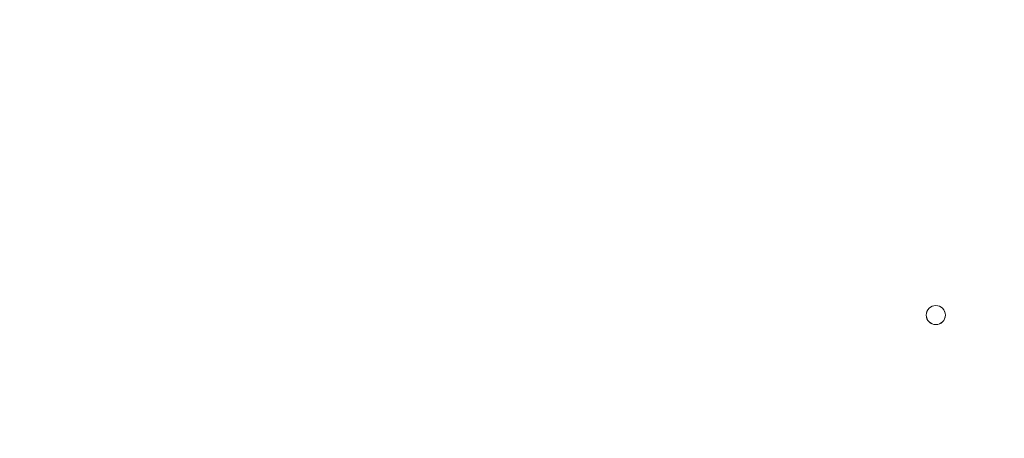
# Model space of a CAD drawing. Units: inches. Extents: x -466983 to 1020, y 324 to 318697.
# Tile 56 of 97: x 637.858 to 643.839, y 936.436 to 938.98. Entities that reach past the tile are written whole.
import ezdxf

# ---------------------------------------------------------------- set-up
doc = ezdxf.new("R2010")
doc.units = ezdxf.units.IN
doc.header["$MEASUREMENT"] = 0
doc.layers.add('A-FLOR-PATT', color=252, linetype='Continuous', lineweight=13)
doc.layers.add('A-FURN', color=8, linetype='Continuous', lineweight=18)

# ---------------------------------------------------------------- blocks, each defined once
blk = doc.blocks.new('L Shaped Sofa')
at = {"ltscale": 2}
for start, end in [(90, 270), (270, 90)]:
    blk.add_arc((2419.413, 753.788), 0.106, start, end, dxfattribs=at)

msp = doc.modelspace()

# ---------------------------------------------------------------- hatches: boundary and pattern name
at = {"layer": 'A-FLOR-PATT', "transparency": 33554572}
h = msp.add_hatch(dxfattribs=at)
h.set_pattern_fill('ANSI37', color=256, scale=30)
h.set_pattern_definition([(45, (-1212.4137, -290.035), (-2.6516504, 2.6516504), []), (135, (-1212.4137, -290.035), (-2.6516504, -2.6516504), [])])
h.paths.add_polyline_path([(901.8057, 1075.9377), (900.6144, 1075.9377), (900.6144, 1065.3856), (899.391, 1065.3856), (898.0911, 1065.3856), (892.8356, 1058.7098, -0.258377), (892.1875, 1058.3509), (879.9848, 1058.3509, -0.20177), (879.4382, 1058.5808), (874.0812, 1065.3856), (872.7813, 1065.3856), (871.5579, 1065.3856), (871.5579, 1075.9377), (813.8057, 1075.9377), (813.8057, 1044.7922), (832.3947, 1044.7922, -0.394795), (848.6602, 1028.5356), (848.6602, 1009.9377), (901.8057, 1009.9377), (901.8057, 1015.9377), (901.3057, 1015.9377), (871.3057, 1015.9377), (871.3057, 1017.2502), (871.3344, 1017.2502, -0.401453), (901.3057, 1045.9377), (901.8057, 1045.9377)])
edge = h.paths.add_edge_path(flags=16)
edge.add_line((847.7731, 1068.9486), (847.7731, 1073.7088))
edge.add_arc((849.2269, 1073.7088), 1.4538, 90, 180, ccw=False)
edge.add_line((849.2269, 1075.1627), (864.4921, 1075.1627))
edge.add_arc((864.4921, 1073.7088), 1.4538, 0, 90, ccw=False)
edge.add_line((865.9459, 1073.7088), (865.9459, 1069.0035))
edge.add_arc((832.6447, 1068.9761), 33.3012, -20.61234, 0.04725, ccw=False)
edge.add_ellipse((856.8595, 1058.48), major_axis=(0, 10.2131), ratio=0.6859192, start_angle=100.00884, end_angle=259.99116, ccw=False)
edge.add_arc((881.0742, 1068.9761), 33.3012, 180.04725, 200.61234, ccw=False)
h.paths.add_polyline_path([(853.1456, 1066.4815), (853.1456, 1066.4534), (853.1463, 1066.4534, 0.433107), (852.9166, 1066.6849), (852.9166, 1066.4534), (853.1456, 1066.4534), (853.1456, 1066.4815), (853.088, 1066.6122, 0.697939), (852.6995, 1066.4534), (852.7003, 1066.4534), (852.7003, 1066.4815), (852.9166, 1067.0012), (852.9166, 1066.6849, -0.396254)], flags=0)
h.paths.add_polyline_path([(861.0187, 1066.4815), (861.0187, 1066.4534), (861.0194, 1066.4534, 0.416404), (860.8024, 1066.6849), (860.8024, 1066.4534), (861.0187, 1066.4534), (861.0187, 1066.4815), (860.9672, 1066.6053, 0.713344), (860.5726, 1066.4534), (860.5734, 1066.4534), (860.5734, 1066.4815), (860.8024, 1067.0012), (860.8024, 1066.6849, -0.379973)], flags=0)
edge = h.paths.add_edge_path(flags=0)
edge.add_spline(control_points=[(861.1298, 1065.7855), (861.4661, 1065.2478), (861.6134, 1065.0161), (861.9833, 1064.3736), (862.1924, 1063.9443), (862.5614, 1063.0391), (862.7212, 1062.5633), (862.9865, 1061.5781), (863.092, 1061.0689), (863.2452, 1060.031), (863.293, 1059.5025), (863.3295, 1058.4409), (863.3181, 1057.9078), (863.2366, 1056.8518), (863.1664, 1056.3289), (862.9695, 1055.308), (862.8427, 1054.8099), (862.5365, 1053.8522), (862.3571, 1053.3927), (861.9514, 1052.5249), (861.7251, 1052.1166), (861.233, 1051.3622), (860.9672, 1051.0162), (860.4048, 1050.3949), (860.1082, 1050.1197), (859.4937, 1049.6461), (859.1758, 1049.4476), (858.5276, 1049.1299), (858.1973, 1049.0107), (857.5315, 1048.8518), (857.1959, 1048.8121), (856.5249, 1048.812), (856.1894, 1048.8515), (855.5236, 1049.0101), (855.1933, 1049.1291), (854.545, 1049.4465), (854.2271, 1049.6449), (853.6124, 1050.1183), (853.3158, 1050.3933), (852.7533, 1051.0143), (852.4874, 1051.3602), (851.9952, 1052.1144), (851.7688, 1052.5225), (851.3629, 1053.3902), (851.1834, 1053.8496), (850.877, 1054.8071), (850.7501, 1055.3051), (850.553, 1056.326), (850.4827, 1056.8488), (850.401, 1057.9048), (850.3895, 1058.4379), (850.4257, 1059.4995), (850.4734, 1060.0281), (850.6265, 1061.066), (850.7318, 1061.5753), (850.9969, 1062.5605), (851.1567, 1063.0365), (851.5254, 1063.9418), (851.7345, 1064.3712), (852.1056, 1065.0164), (852.2544, 1065.2503), (852.6082, 1065.7335)], knot_values=[3.915332, 3.915332, 3.915332, 3.915332, 4.013468, 4.013468, 4.175532, 4.175532, 4.337596, 4.337596, 4.49966, 4.49966, 4.661724, 4.661724, 4.823788, 4.823788, 4.985852, 4.985852, 5.147916, 5.147916, 5.30998, 5.30998, 5.472044, 5.472044, 5.634109, 5.634109, 5.796173, 5.796173, 5.958237, 5.958237, 6.120301, 6.120301, 6.282365, 6.282365, 6.444429, 6.444429, 6.606493, 6.606493, 6.768557, 6.768557, 6.930621, 6.930621, 7.092685, 7.092685, 7.254749, 7.254749, 7.416813, 7.416813, 7.578878, 7.578878, 7.740942, 7.740942, 7.903006, 7.903006, 8.06507, 8.06507, 8.227134, 8.227134, 8.389198, 8.389198, 8.551262, 8.551262, 8.65037, 8.65037, 8.65037, 8.65037], degree=3, periodic=0)
edge.add_line((852.6421, 1065.7855), (861.1298, 1065.7855))
edge = h.paths.add_edge_path(flags=0)
edge.add_ellipse((856.8496, 1057.7432), major_axis=(0, 7.7921), ratio=0.687861, start_angle=0, end_angle=360)
h.paths.add_polyline_path([(848.8634, 1069.3891), (848.8634, 1073.9605, -0.414214), (849.9538, 1075.0508), (863.7652, 1075.0508, -0.414214), (864.8555, 1073.9605), (864.8555, 1069.3891, -0.388936), (864.5237, 1069.027, -0.043561), (849.1953, 1069.027, -0.388936)], flags=0)
h.paths.add_polyline_path([(853.1006, 1068.1122, -1), (852.6775, 1068.1122, -1)], flags=0)
edge = h.paths.add_edge_path(flags=0)
edge.add_ellipse((856.8595, 1057.3378), major_axis=(0, 2.207), ratio=0.657164, start_angle=0, end_angle=360)
h.paths.add_polyline_path([(861.0415, 1068.1122, -1), (860.6184, 1068.1122, -1)], flags=0)
edge = h.paths.add_edge_path()
edge.add_line((573.9537, 1057.3412), (573.9537, 1075.9377))
edge.add_line((573.9537, 1075.9377), (558.7308, 1075.9377))
edge.add_line((558.7308, 1075.9377), (558.7308, 1065.3856))
edge.add_line((558.7308, 1065.3856), (557.5074, 1065.3856))
edge.add_line((557.5074, 1065.3856), (556.2075, 1065.3856))
edge.add_line((556.2075, 1065.3856), (550.952, 1058.7098))
edge.add_arc((550.3039, 1059.1155), 0.7646, 270, 327.94832, ccw=False)
edge.add_line((550.3039, 1058.3509), (538.1012, 1058.3509))
edge.add_arc((538.1012, 1059.1155), 0.7646, 224.3704, 270, ccw=False)
edge.add_line((537.5546, 1058.5808), (532.1976, 1065.3856))
edge.add_line((532.1976, 1065.3856), (530.8977, 1065.3856))
edge.add_line((530.8977, 1065.3856), (529.6743, 1065.3856))
edge.add_line((529.6743, 1065.3856), (529.6743, 1075.9377))
edge.add_line((529.6743, 1075.9377), (520.8057, 1075.9377))
edge.add_line((520.8057, 1075.9377), (520.8057, 1045.9377))
edge.add_line((520.8057, 1045.9377), (521.3057, 1045.9377))
edge.add_arc((521.3057, 1015.9377), 30, 2.50749, 90, ccw=False)
edge.add_line((551.277, 1017.2502), (551.3057, 1017.2502))
edge.add_line((551.3057, 1017.2502), (551.3057, 1015.9377))
edge.add_line((551.3057, 1015.9377), (520.8057, 1015.9377))
edge.add_line((520.8057, 1015.9377), (520.8057, 1009.9377))
edge.add_line((520.8057, 1009.9377), (559.1913, 1010.4022))
edge.add_arc((559.1913, 1011.856), 1.4538, 180, 270, ccw=False)
edge.add_line((557.7375, 1011.856), (557.7375, 1016.5613))
edge.add_arc((591.0386, 1016.5888), 33.3012, 159.38766, 180.04725, ccw=False)
edge.add_ellipse((566.8239, 1027.0848), major_axis=(0, 10.2131), ratio=0.6859192, start_angle=280.00884, end_angle=439.99116, ccw=False)
edge.add_arc((542.6091, 1016.5888), 33.3012, 0.04725, 20.61234, ccw=False)
edge.add_line((575.9103, 1016.6162), (575.9103, 1011.856))
edge.add_arc((574.4565, 1011.856), 1.4538, -90, 0, ccw=False)
edge.add_line((574.4565, 1010.4022), (608.8057, 1009.9377))
edge.add_line((608.8057, 1009.9377), (608.8057, 1041.0857))
edge.add_line((608.8057, 1041.0857), (590.2179, 1041.0857))
edge.add_arc((590.775, 1057.9074), 16.8309, 181.92775, 268.10321, ccw=False)
edge = h.paths.add_edge_path()
edge.add_ellipse((494.2443, 583.6204), major_axis=(0, 10.2131), ratio=0.6859192, start_angle=280.00884, end_angle=439.99116, ccw=False)
edge.add_arc((470.0296, 573.1243), 33.3012, 0.04725, 20.61234, ccw=False)
edge.add_line((503.3307, 573.1518), (503.3307, 568.3916))
edge.add_arc((501.8769, 568.3916), 1.4538, -90, 0, ccw=False)
edge.add_line((501.8769, 566.9377), (539.8057, 566.9377))
edge.add_line((539.8057, 566.9377), (539.8057, 572.9377))
edge.add_line((539.8057, 572.9377), (539.3057, 572.9377))
edge.add_line((539.3057, 572.9377), (509.3057, 572.9377))
edge.add_line((509.3057, 572.9377), (509.3057, 574.2502))
edge.add_line((509.3057, 574.2502), (509.3344, 574.2502))
edge.add_arc((539.3057, 572.9377), 30, 90, 177.49251, ccw=False)
edge.add_line((539.3057, 602.9377), (539.8057, 602.9377))
edge.add_line((539.8057, 602.9377), (539.8057, 626.9377))
edge.add_line((539.8057, 626.9377), (531.7718, 626.9377))
edge.add_line((531.7718, 626.9377), (531.7718, 616.3856))
edge.add_line((531.7718, 616.3856), (530.5484, 616.3856))
edge.add_line((530.5484, 616.3856), (529.2485, 616.3856))
edge.add_line((529.2485, 616.3856), (523.7105, 609.3509))
edge.add_line((523.7105, 609.3509), (510.7766, 609.3509))
edge.add_line((510.7766, 609.3509), (505.2386, 616.3856))
edge.add_line((505.2386, 616.3856), (503.9387, 616.3856))
edge.add_line((503.9387, 616.3856), (502.7153, 616.3856))
edge.add_line((502.7153, 616.3856), (502.7153, 626.9377))
edge.add_line((502.7153, 626.9377), (481.6983, 626.9377))
edge.add_line((481.6983, 626.9377), (481.6983, 610.995))
edge.add_arc((467.2703, 611.4728), 14.4359, 271.92775, 358.10321, ccw=False)
edge.add_line((467.7559, 597.0451), (451.8057, 597.0451))
edge.add_line((451.8057, 597.0451), (451.8057, 584.4035))
edge.add_line((451.8057, 584.4035), (451.8057, 566.9377))
edge.add_line((451.8057, 566.9377), (486.6117, 566.9377))
edge.add_arc((486.6117, 568.3916), 1.4538, 180, 270, ccw=False)
edge.add_line((485.1579, 568.3916), (485.1579, 573.0969))
edge.add_arc((518.4591, 573.1243), 33.3012, 159.38766, 180.04725, ccw=False)
h.paths.add_polyline_path([(836.2609, 1020.7328), (879.8898, 1020.7328), (879.8898, 1039.3902), (836.2609, 1039.3902)], flags=25)
h.paths.add_polyline_path([(549.9851, 1036.7492), (593.614, 1036.7492), (593.614, 1055.4065), (549.9851, 1055.4065)], flags=24)
h.paths.add_polyline_path([(475.123, 595.5959), (518.752, 595.5959), (518.752, 614.2532), (475.123, 614.2532)], flags=24)
h = msp.add_hatch(dxfattribs=at)
h.set_pattern_fill('ANSI37', color=256, scale=20)
h.set_pattern_definition([(45, (-1212.4137, -290.035), (-1.767767, 1.767767), []), (135, (-1212.4137, -290.035), (-1.767767, -1.767767), [])])
h.paths.add_polyline_path([(809.8057, 870.9377), (809.8057, 888.1519), (806.9985, 888.1519), (802.6624, 888.1519), (789.3832, 888.1519), (786.2846, 888.1519, -0.414214), (785.4991, 888.9374), (785.4991, 900.1959), (785.4991, 908.4696, -0.414214), (786.8082, 909.7787, -0.414214), (785.4991, 911.0878), (785.4991, 929.1015, -0.414214), (786.8082, 930.4106, -0.414214), (785.4991, 931.7197), (785.4991, 931.9039, -0.414214), (784.19, 930.5948), (766.7223, 930.5948, -0.412359), (765.4132, 931.8956, -0.413741), (764.1145, 930.5782), (744.5781, 930.422, -0.416556), (743.7864, 931.2075), (743.7864, 933.5153), (742.2154, 933.5153), (742.2154, 952.024, -0.001344), (743.7864, 952.1998), (743.7864, 953.9377), (678.5915, 953.9377), (678.5915, 951.1305), (678.5915, 946.7945), (678.5915, 933.5153), (678.5915, 930.4166, -0.414214), (677.806, 929.6312), (666.5475, 929.6312), (658.2738, 929.6312, -0.414214), (656.9647, 930.9403, -0.414214), (655.6556, 929.6312), (637.6419, 929.6312, -0.414214), (636.3328, 930.9403, -0.414214), (635.0237, 929.6312), (634.8395, 929.6312, -0.414214), (636.1486, 928.322), (636.1486, 910.8544, -0.412359), (634.8478, 909.5452, -0.413741), (636.1653, 908.2466), (636.3214, 888.7102, -0.416556), (635.5359, 887.9184), (633.2281, 887.9184), (633.2281, 886.3475), (614.7194, 886.3475, -0.001344), (614.5436, 887.9184), (612.8057, 887.9184), (612.8057, 834.9377), (612.8057, 752.9377), (612.8057, 748.9377), (612.8057, 697.9377), (654.8057, 697.9377), (654.8057, 701.9377), (715.8057, 701.9377), (715.8057, 737.4353), (774.2918, 737.4353), (774.2918, 795.9377), (809.8057, 795.9377)])
h.paths.add_polyline_path([(679.2761, 849.5757, 0.102523), (682.1475, 849.2608, -0.080461), (694.5428, 849.7725, -0.283899), (694.4822, 849.0082, 0.136605), (694.4068, 848.8103, -0.030441), (694.5428, 846.8929), (694.5428, 842.6198), (694.5428, 838.3466, -0.028219), (694.4246, 836.5684), (694.425, 836.5684, 0.196187), (694.4456, 836.2708, -0.302897), (694.5428, 835.467, -0.080461), (682.1475, 835.9787, 0.102523), (679.2761, 835.6638, -0.58611), (678.6457, 836.0169), (678.6457, 849.2227, -0.58611)], flags=16)
h.paths.add_polyline_path([(679.5173, 848.6515, 0.699597), (679.476, 848.6342, 1.20716), (679.1935, 848.7422, 0.010621)], flags=0)
h.paths.add_polyline_path([(679.4923, 836.5608, -0.013798), (679.9178, 836.6594, -0.071703), (682.8533, 837.1434, -0.165743), (682.1665, 839.1006), (682.1665, 842.6094), (682.1665, 846.0603, -0.240616), (683.4733, 848.6767, -0.068263), (693.9295, 849.0082), (693.7875, 848.7083), (693.7875, 849.0228, 0.067332), (683.4733, 848.6767, 0.240616), (682.1665, 846.0603), (682.1665, 842.6094), (682.1665, 839.1006, 0.23459), (683.461, 836.5513, 0.068093), (693.7875, 836.1955), (693.7875, 836.5104), (693.9296, 836.2102, -0.077215), (682.2421, 836.7815, 0.086627), (679.5283, 836.5701, -0.628402), (679.5029, 836.5735), (679.5029, 836.6071, 0.910458)], flags=0)
h.paths.add_polyline_path([(679.476, 848.6364), (679.2069, 848.647), (679.2069, 836.5718, 0.913566), (679.3645, 836.5861), (679.476, 836.5824)], flags=0)
h.paths.add_polyline_path([(679.2761, 829.8604, 0.102523), (682.1475, 829.5455, -0.080461), (694.5428, 830.0572, -0.283899), (694.4822, 829.2929, 0.136605), (694.4068, 829.095, -0.030441), (694.5428, 827.1776), (694.5428, 822.9045), (694.5428, 818.6314, -0.028219), (694.4246, 816.8531), (694.425, 816.8532, 0.196187), (694.4456, 816.5555, -0.302897), (694.5428, 815.7517, -0.080461), (682.1475, 816.2635, 0.102523), (679.2761, 815.9485, -0.58611), (678.6457, 816.3016), (678.6457, 829.5074, -0.58611)], flags=16)
h.paths.add_polyline_path([(679.5173, 828.9362, 0.699597), (679.476, 828.9189, 1.20716), (679.1935, 829.0269, 0.010621)], flags=0)
h.paths.add_polyline_path([(679.4923, 816.8456, -0.013798), (679.9178, 816.9441, -0.071703), (682.8533, 817.4281, -0.165743), (682.1665, 819.3853), (682.1665, 822.8941), (682.1665, 826.345, -0.240616), (683.4733, 828.9614, -0.068263), (693.9295, 829.2929), (693.7875, 828.9931), (693.7875, 829.3076, 0.067332), (683.4733, 828.9614, 0.240616), (682.1665, 826.345), (682.1665, 822.8941), (682.1665, 819.3853, 0.23459), (683.461, 816.836, 0.068093), (693.7875, 816.4802), (693.7875, 816.7952), (693.9296, 816.4949, -0.077215), (682.2421, 817.0662, 0.086627), (679.5283, 816.8549, -0.628402), (679.5029, 816.8582), (679.5029, 816.8918, 0.910458)], flags=0)
h.paths.add_polyline_path([(679.476, 828.9211), (679.2069, 828.9317), (679.2069, 816.8565, 0.913566), (679.3645, 816.8708), (679.476, 816.8671)], flags=0)
h.paths.add_polyline_path([(679.2761, 810.1451, 0.102523), (682.1475, 809.8302, -0.080461), (694.5428, 810.342, -0.3023), (694.4466, 809.5394, 0.10023), (694.4058, 809.3878, -0.03057), (694.5428, 807.4623), (694.5428, 803.1892), (694.5428, 798.9161, -0.03057), (694.4058, 796.9906, 0.10023), (694.4466, 796.839, -0.3023), (694.5428, 796.0365, -0.080461), (682.1475, 796.5482, 0.102523), (679.2761, 796.2333, -0.58611), (678.6457, 796.5863), (678.6457, 809.7921, -0.58611)], flags=16)
h.paths.add_polyline_path([(679.5173, 809.2417, 0.699597), (679.476, 809.2244, 1.20716), (679.1935, 809.3324, 0.010621)], flags=0)
h.paths.add_polyline_path([(679.4923, 797.151, -0.013798), (679.9178, 797.2496, -0.071703), (682.8533, 797.7336, -0.165743), (682.1665, 799.6908), (682.1665, 803.1996), (682.1665, 806.6505, -0.239349), (683.461, 809.2577, -0.072465), (694.4468, 809.5405, 0.197932), (694.425, 809.2405), (693.7875, 809.2985), (693.7875, 809.6135, 0.068093), (683.461, 809.2577, 0.239349), (682.1665, 806.6505), (682.1665, 803.1996), (682.1665, 799.6908, 0.235854), (683.4733, 797.1323, 0.067332), (693.7875, 796.7861), (693.7875, 797.1006), (694.425, 797.1586, 0.197932), (694.4468, 796.8586, -0.080419), (682.1557, 797.3795, 0.083867), (679.5283, 797.1603, -0.628402), (679.5029, 797.1637), (679.5029, 797.1973, 0.910458)], flags=0)
h.paths.add_polyline_path([(679.2069, 809.2372), (679.2069, 797.162, 0.913566), (679.3645, 797.1763), (679.476, 797.1726), (679.476, 809.2266)], flags=0)
h.paths.add_polyline_path([(695.3643, 853.2989), (728.2231, 853.2989), (728.2231, 771.1519), (695.3643, 771.1519)], flags=16)
h.paths.add_polyline_path([(696.0215, 852.6417), (727.5659, 852.6417), (727.5659, 771.809), (696.0215, 771.809)], flags=0)
h.paths.add_polyline_path([(679.2761, 788.7869, 0.102523), (682.1475, 788.472, -0.080461), (694.5428, 788.9837, -0.3023), (694.4466, 788.1812, 0.10023), (694.4058, 788.0296, -0.03057), (694.5428, 786.1041), (694.5428, 781.831), (694.5428, 777.5578, -0.03057), (694.4058, 775.6323, 0.10023), (694.4466, 775.4808, -0.3023), (694.5428, 774.6782, -0.080461), (682.1475, 775.19, 0.102523), (679.2761, 774.875, -0.58611), (678.6457, 775.2281), (678.6457, 788.4339, -0.58611)], flags=16)
h.paths.add_polyline_path([(679.5173, 787.8834, 0.699597), (679.476, 787.8662, 1.20716), (679.1935, 787.9742, 0.010621)], flags=0)
h.paths.add_polyline_path([(679.4923, 775.7928, -0.013798), (679.9178, 775.8914, -0.071703), (682.8533, 776.3753, -0.165743), (682.1665, 778.3325), (682.1665, 781.8414), (682.1665, 785.2922, -0.239349), (683.461, 787.8995, -0.072465), (694.4468, 788.1823, 0.197932), (694.425, 787.8823), (693.7875, 787.9403), (693.7875, 788.2553, 0.068093), (683.461, 787.8995, 0.239349), (682.1665, 785.2922), (682.1665, 781.8414), (682.1665, 778.3325, 0.235854), (683.4733, 775.7741, 0.067332), (693.7875, 775.4279), (693.7875, 775.7424), (694.425, 775.8004, 0.197932), (694.4468, 775.5004, -0.080419), (682.1557, 776.0212, 0.083867), (679.5283, 775.8021, -0.628402), (679.5029, 775.8054), (679.5029, 775.8391, 0.910458)], flags=0)
h.paths.add_polyline_path([(679.2069, 787.8789), (679.2069, 775.8038, 0.913566), (679.3645, 775.818), (679.476, 775.8144), (679.476, 787.8684)], flags=0)
h.paths.add_polyline_path([(704.641, 854.1204, -0.080461), (705.1527, 866.5157, 0.102523), (704.8378, 869.3871, -0.58611), (705.1908, 870.0174), (718.3966, 870.0174, -0.58611), (718.7496, 869.3871, 0.102523), (718.4347, 866.5157, -0.080461), (718.9465, 854.1204, -0.3023), (718.1439, 854.2166, 0.10023), (717.9924, 854.2574, -0.03057), (716.0668, 854.1204), (711.7937, 854.1204), (707.5206, 854.1204, -0.03057), (705.5951, 854.2574, 0.10023), (705.4435, 854.2166, -0.3023)], flags=16)
h.paths.add_polyline_path([(717.8462, 869.1459, 0.699597), (717.8289, 869.1872, 1.20716), (717.9369, 869.4697, 0.010621)], flags=0)
h.paths.add_polyline_path([(705.4631, 854.2164, -0.080419), (705.984, 866.5074, 0.083867), (705.7648, 869.1349, -0.628402), (705.7682, 869.1603), (705.8018, 869.1603, 0.910458), (705.7555, 869.1709, -0.013798), (705.8541, 868.7454, -0.071703), (706.3381, 865.8099, -0.165743), (708.2953, 866.4967), (711.8041, 866.4967), (715.255, 866.4967, -0.239349), (717.8622, 865.2022, -0.072465), (718.145, 854.2164, 0.197932), (717.845, 854.2382), (717.903, 854.8757), (718.218, 854.8757, 0.068093), (717.8622, 865.2022, 0.239349), (715.255, 866.4967), (711.8041, 866.4967), (708.2953, 866.4967, 0.235854), (705.7368, 865.1898, 0.067332), (705.3906, 854.8757), (705.7051, 854.8757), (705.7631, 854.2382, 0.197932)], flags=16)
h.paths.add_polyline_path([(705.7665, 869.4563, 0.913566), (705.7808, 869.2987), (705.7771, 869.1872), (717.8311, 869.1872), (717.8417, 869.4563)], flags=0)
h.paths.add_polyline_path([(729.0446, 842.6198), (729.0446, 846.8929, -0.03057), (729.1817, 848.8184, 0.10023), (729.1408, 848.9699, -0.3023), (729.0446, 849.7725, -0.080461), (741.4399, 849.2608, 0.102523), (744.3113, 849.5757, -0.58611), (744.9417, 849.2227), (744.9417, 836.0169, -0.58611), (744.3113, 835.6638, 0.102523), (741.4399, 835.9787, -0.080461), (729.0446, 835.467, -0.3023), (729.1408, 836.2696, 0.10023), (729.1817, 836.4211, -0.03057), (729.0446, 838.3466)], flags=16)
h.paths.add_polyline_path([(744.1115, 836.5846, 1.20716), (744.3939, 836.4766, 0.010621), (744.0701, 836.5673, 0.699597)], flags=0)
h.paths.add_polyline_path([(729.1407, 836.2684, 0.197932), (729.1624, 836.5684), (729.7999, 836.5104), (729.7999, 836.1955, 0.068093), (740.1264, 836.5513, 0.239349), (741.4209, 839.1585), (741.4209, 842.6094), (741.4209, 846.1182, 0.235854), (740.1141, 848.6767, 0.067332), (729.7999, 849.0228), (729.7999, 848.7083), (729.1624, 848.6503, 0.197932), (729.1407, 848.9504, -0.080419), (741.4317, 848.4295, 0.083867), (744.0591, 848.6486, -0.628402), (744.0845, 848.6453), (744.0845, 848.6117, 0.910458), (744.0951, 848.6579, -0.013798), (743.6696, 848.5594, -0.071703), (740.7341, 848.0754, -0.165743), (741.4209, 846.1182), (741.4209, 842.6094), (741.4209, 839.1585, -0.239349), (740.1264, 836.5513, -0.072465)], flags=0)
h.paths.add_polyline_path([(729.0446, 830.0572, -0.080461), (741.4399, 829.5455, 0.102523), (744.3113, 829.8604, -0.58611), (744.9417, 829.5074), (744.9417, 816.3016, -0.58611), (744.3113, 815.9485, 0.102523), (741.4399, 816.2635, -0.080461), (729.0446, 815.7517, -0.3023), (729.1408, 816.5543, 0.10023), (729.1817, 816.7058, -0.03057), (729.0446, 818.6314), (729.0446, 822.9045), (729.0446, 827.1776, -0.03057), (729.1817, 829.1031, 0.10023), (729.1408, 829.2547, -0.3023)], flags=16)
h.paths.add_polyline_path([(744.1115, 816.8693, 1.20716), (744.3939, 816.7613, 0.010621), (744.0701, 816.852, 0.699597)], flags=0)
h.paths.add_polyline_path([(729.1407, 829.2351, -0.080419), (741.4317, 828.7142, 0.083867), (744.0591, 828.9334, -0.628402), (744.0845, 828.93), (744.0845, 828.8964, 0.910458), (744.0951, 828.9427, -0.013798), (743.6696, 828.8441, -0.071703), (740.7341, 828.3601, -0.165743), (741.4209, 826.4029), (741.4209, 822.8941), (741.4209, 819.4432, -0.239349), (740.1264, 816.836, -0.072465), (729.1407, 816.5531, 0.197932), (729.1624, 816.8532), (729.7999, 816.7952), (729.7999, 816.4802, 0.068093), (740.1264, 816.836, 0.239349), (741.4209, 819.4432), (741.4209, 822.8941), (741.4209, 826.4029, 0.235854), (740.1141, 828.9614, 0.067332), (729.7999, 829.3076), (729.7999, 828.9931), (729.1624, 828.9351, 0.197932)], flags=16)
h.paths.add_polyline_path([(729.0446, 810.342, -0.080461), (741.4399, 809.8302, 0.102523), (744.3113, 810.1451, -0.58611), (744.9417, 809.7921), (744.9417, 796.5863, -0.58611), (744.3113, 796.2333, 0.102523), (741.4399, 796.5482, -0.080461), (729.0446, 796.0365, -0.283899), (729.1052, 796.8007, 0.136605), (729.1806, 796.9987, -0.030441), (729.0446, 798.9161), (729.0446, 803.1892), (729.0446, 807.4623, -0.028219), (729.1628, 809.2406), (729.1624, 809.2405, 0.196187), (729.1418, 809.5382, -0.302897)], flags=16)
h.paths.add_polyline_path([(744.1115, 797.1748, 1.20716), (744.3939, 797.0668, 0.010621), (744.0701, 797.1575, 0.699597)], flags=0)
h.paths.add_polyline_path([(741.3453, 809.0275, 0.086627), (744.0591, 809.2388, -0.628402), (744.0845, 809.2355), (744.0845, 809.2019, 0.910458), (744.0951, 809.2481, -0.013798), (743.6696, 809.1496, -0.071703), (740.7341, 808.6656, -0.165743), (741.4209, 806.7084), (741.4209, 803.1996), (741.4209, 799.7487, -0.240616), (740.1141, 797.1323, -0.068263), (729.658, 796.8008), (729.7999, 797.1006), (729.7999, 796.7861, 0.067332), (740.1141, 797.1323, 0.240616), (741.4209, 799.7487), (741.4209, 803.1996), (741.4209, 806.7084, 0.23459), (740.1264, 809.2577, 0.068093), (729.7999, 809.6135), (729.7999, 809.2985), (729.6578, 809.5988, -0.077215)], flags=0)
h.paths.add_polyline_path([(704.641, 770.3304, -0.283899), (705.4053, 770.2697, 0.136605), (705.6032, 770.1944, -0.030441), (707.5206, 770.3304), (711.7937, 770.3304), (716.0668, 770.3304, -0.028219), (717.8451, 770.2122), (717.845, 770.2126, 0.196187), (718.1427, 770.2331, -0.302897), (718.9465, 770.3304, -0.080461), (718.4347, 757.9351, 0.102523), (718.7496, 755.0637, -0.58611), (718.3966, 754.4333), (705.1908, 754.4333, -0.58611), (704.8378, 755.0637, 0.102523), (705.1527, 757.9351, -0.080461)], flags=16)
h.paths.add_polyline_path([(705.762, 755.3048, 0.699597), (705.7793, 755.2635, 1.20716), (705.6713, 754.9811, 0.010621)], flags=0)
h.paths.add_polyline_path([(705.4053, 769.717), (705.7051, 769.5751), (705.3906, 769.5751, 0.067332), (705.7368, 759.2609, 0.240616), (708.3532, 757.954), (711.8041, 757.954), (715.3129, 757.954, 0.23459), (717.8622, 759.2485, 0.068093), (718.218, 769.5751), (717.903, 769.5751), (718.2033, 769.7172, -0.077215), (717.632, 758.0297, 0.086627), (717.8433, 755.3159, -0.628402), (717.84, 755.2904), (717.8064, 755.2904, 0.910458), (717.8526, 755.2799, -0.013798), (717.7541, 755.7053, -0.071703), (717.2701, 758.6409, -0.165743), (715.3129, 757.954), (711.8041, 757.954), (708.3532, 757.954, -0.240616), (705.7368, 759.2609, -0.068263)], flags=0)
h.paths.add_polyline_path([(729.0446, 788.9837, -0.080461), (741.4399, 788.472, 0.102523), (744.3113, 788.7869, -0.58611), (744.9417, 788.4339), (744.9417, 775.2281, -0.58611), (744.3113, 774.875, 0.102523), (741.4399, 775.19, -0.080461), (729.0446, 774.6782, -0.283899), (729.1052, 775.4425, 0.136605), (729.1806, 775.6405, -0.030441), (729.0446, 777.5578), (729.0446, 781.831), (729.0446, 786.1041, -0.028219), (729.1628, 787.8823), (729.1624, 787.8823, 0.196187), (729.1418, 788.1799, -0.302897)], flags=16)
h.paths.add_polyline_path([(744.1115, 775.8165, 1.20716), (744.3939, 775.7086, 0.010621), (744.0701, 775.7993, 0.699597)], flags=0)
h.paths.add_polyline_path([(741.3453, 787.6692, 0.086627), (744.0591, 787.8806, -0.628402), (744.0845, 787.8773), (744.0845, 787.8437, 0.910458), (744.0951, 787.8899, -0.013798), (743.6696, 787.7913, -0.071703), (740.7341, 787.3074, -0.165743), (741.4209, 785.3502), (741.4209, 781.8414), (741.4209, 778.3905, -0.240616), (740.1141, 775.7741, -0.068263), (729.658, 775.4425), (729.7999, 775.7424), (729.7999, 775.4279, 0.067332), (740.1141, 775.7741, 0.240616), (741.4209, 778.3905), (741.4209, 781.8414), (741.4209, 785.3502, 0.23459), (740.1264, 787.8995, 0.068093), (729.7999, 788.2553), (729.7999, 787.9403), (729.6578, 788.2405, -0.077215)], flags=0)
h.paths.add_polyline_path([(744.1115, 848.6364), (744.1115, 836.5824), (744.3805, 836.5718), (744.3805, 848.647, 0.913566), (744.2229, 848.6327)], flags=0)
h.paths.add_polyline_path([(744.2229, 828.9174), (744.1115, 828.9211), (744.1115, 816.8671), (744.3805, 816.8565), (744.3805, 828.9317, 0.913566)], flags=0)
h.paths.add_polyline_path([(717.8311, 755.2635), (705.7771, 755.2635), (705.7665, 754.9945), (717.8417, 754.9945, 0.913566), (717.8274, 755.1521)], flags=0)
h.paths.add_polyline_path([(744.2229, 809.2229), (744.1115, 809.2266), (744.1115, 797.1726), (744.3805, 797.162), (744.3805, 809.2372, 0.913566)], flags=0)
h.paths.add_polyline_path([(744.1115, 787.8684), (744.1115, 775.8144), (744.3805, 775.8038), (744.3805, 787.8789, 0.913566), (744.2229, 787.8647)], flags=0)
h.paths.add_polyline_path([(678.8774, 877.1228), (737.6127, 877.1228), (737.6127, 899.5116), (678.8774, 899.5116)], flags=24)

# ---------------------------------------------------------------- linework, layer by layer
at = {"layer": 'A-FURN', "ltscale": 2}
for start, end in [(90, 270), (90, 270), (90, 270), (90, 270), (90, 270), (90, 270), (270, 90), (270, 90), (270, 90), (270, 90), (270, 90), (270, 90)]:
    msp.add_arc((643.4233, 937.1848), 0.0582, start, end, dxfattribs=at)

# ---------------------------------------------------------------- block references
at = {"layer": 'A-FURN', "xscale": 0.5482153745360612, "yscale": 0.5482153745360612, "zscale": 0.5482153745360612, "rotation": 180}
msp.add_blockref('L Shaped Sofa', (1969.7828, 1350.4232), dxfattribs=at)

doc.saveas('drawing.dxf')
